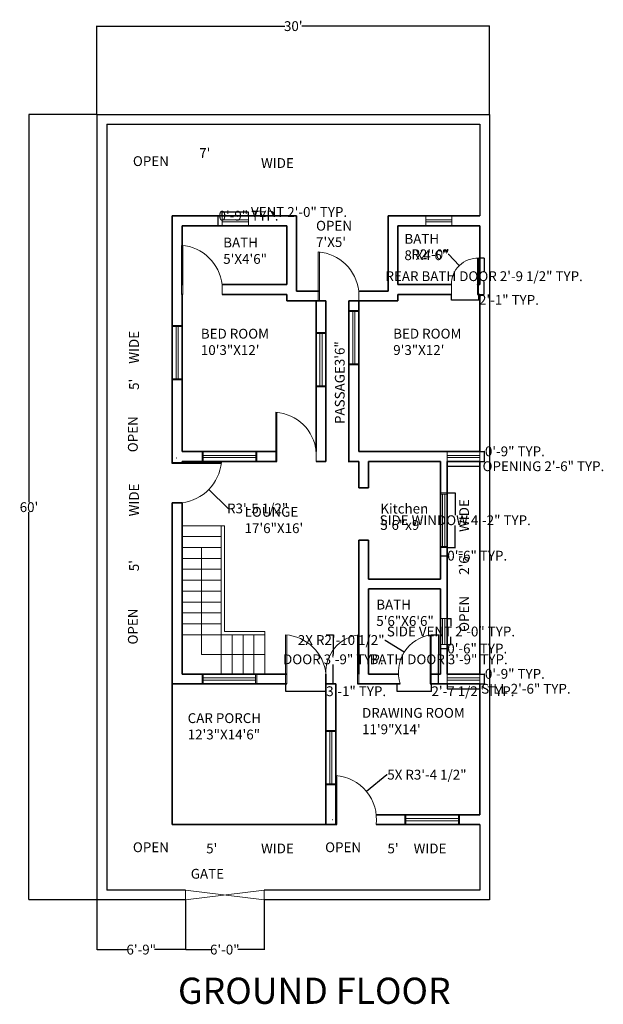
# Model space of a CAD drawing. Units: inches. Extents: x -56 to 1055, y -798 to 815.
# Tile 1 of 2: x -56 to 479, y -798 to 105. Entities that reach past the tile are written whole.
import ezdxf

# ---------------------------------------------------------------- set-up
doc = ezdxf.new("R2010")
doc.units = ezdxf.units.IN
doc.header["$MEASUREMENT"] = 0
for name, color, linetype, lineweight in [('A-ANNO-DIMS', 2, 'Continuous', 18), ('A-ANNO-TEXT', 7, 'Continuous', 18), ('A-AREA-IDEN', 7, 'Continuous', 18), ('A-DOOR', 3, 'Continuous', 18), ('A-FLOR-STRS', 7, 'Continuous', 18), ('A-GLAZ', 4, 'Continuous', 18), ('A-WALL', 7, 'Continuous', 35), ('C-PROP', 8, 'Continuous', 25), ('C-SITE-GATE', 3, 'Continuous', 18)]:
    doc.layers.add(name, color=color, linetype=linetype, lineweight=lineweight)
doc.styles.get("Standard").update_dxf_attribs({"font": 'arial.ttf'})
doc.dimstyles.get("Standard").update_dxf_attribs({"dimtxt": 9, "dimasz": 0.18, "dimexe": 0.18, "dimexo": 0.0625, "dimgap": 0.09, "dimtad": 0, "dimtih": 1, "dimtoh": 1, "dimdec": 0, "dimzin": 0, "dimdsep": 46, "dimlunit": 3, "dimtxsty": 'Standard', "dimcen": 0.09, "dimadec": 0, "dimazin": 0, "dimtfac": 1, "dimtdec": 0, "dimtofl": 0, "dimtmove": 0, "dimatfit": 3, "dimfxl": 1, "dimtolj": 1, "dimtzin": 0, "dimarcsym": 0})

# ---------------------------------------------------------------- blocks, each defined once
blk = doc.blocks.new('door')
for p, q in [((432.11, -633.03), (432.11, -588.03)), ((433.11, -633.03), (433.11, -588.03)), ((469.11, -624.03), (469.11, -633.03))]:
    blk.add_line(p, q)
blk.add_arc((428.9, -628.35), 40.45, 6.12759, 85.44206)
blk = doc.blocks.new('*D2')
at = {"layer": 'A-ANNO-DIMS', "color": 0, "lineweight": -2, "transparency": 16777216}
for p, q in [((15.17, 18.03), (15.17, 99.11)), ((15.35, 98.93), (187.44, 98.93)), ((374.99, 98.93), (202.89, 98.93)), ((375.17, 18.03), (375.17, 99.11))]:
    blk.add_line(p, q, dxfattribs=at)
at = {"layer": 'A-ANNO-DIMS', "color": 0, "transparency": 16777216}
for points in [[(15.35, 98.96), (15.35, 98.9), (15.17, 98.93)], [(374.99, 98.96), (374.99, 98.9), (375.17, 98.93)]]:
    blk.add_solid(points, dxfattribs=at)
at = {"layer": 'Defpoints', "color": 0, "transparency": 16777216}
for p in [(375.17, 98.93), (15.17, 17.97), (375.17, 17.97)]:
    blk.add_point(p, dxfattribs=at)
at = {"layer": 'A-ANNO-DIMS', "color": 0, "transparency": 16777216, "insert": (195.17, 98.93), "char_height": 9, "attachment_point": 5}
blk.add_mtext("\\A1;30'", dxfattribs=at)
blk = doc.blocks.new('*D3')
at = {"layer": 'A-ANNO-DIMS', "color": 0, "lineweight": -2, "transparency": 16777216}
for p, q in [((15.1, 17.97), (-47.33, 17.97)), ((-47.15, 17.79), (-47.15, -337.35)), ((-47.15, -701.85), (-47.15, -346.72)), ((15.1, -702.03), (-47.33, -702.03))]:
    blk.add_line(p, q, dxfattribs=at)
at = {"layer": 'A-ANNO-DIMS', "color": 0, "transparency": 16777216}
for points in [[(-47.18, 17.79), (-47.12, 17.79), (-47.15, 17.97)], [(-47.18, -701.85), (-47.12, -701.85), (-47.15, -702.03)]]:
    blk.add_solid(points, dxfattribs=at)
at = {"layer": 'Defpoints', "color": 0, "transparency": 16777216}
for p in [(-47.15, 17.97), (15.17, 17.97), (15.17, -702.03)]:
    blk.add_point(p, dxfattribs=at)
at = {"layer": 'A-ANNO-DIMS', "color": 0, "transparency": 16777216, "insert": (-47.15, -342.03), "char_height": 9, "attachment_point": 5}
blk.add_mtext("\\A1;60'", dxfattribs=at)
blk = doc.blocks.new('WIN-50-FRAMED')
for p, q in [((0, 50), (9, 50)), ((0, 0), (0, 50)), ((0, 49), (9, 49)), ((3.5, 1), (3.5, 49)), ((5.5, 1), (5.5, 49)), ((9, 0), (9, 50)), ((0, 1), (9, 1)), ((0, 0), (9, 0))]:
    blk.add_line(p, q)
blk = doc.blocks.new('WIN-50-JAMB')
for p, q in [((0, 0), (0, 9)), ((1, 0), (1, 9)), ((1, 5.5), (49, 5.5)), ((1, 3.5), (49, 3.5)), ((49, 0), (49, 9)), ((50, 0), (50, 9))]:
    blk.add_line(p, q)
blk = doc.blocks.new('WIN-50-NARROW-WALL')
for p, q in [((0, 50), (6, 50)), ((0, 49), (6, 49)), ((2, 49), (2, 1)), ((4, 49), (4, 1)), ((0, 1), (6, 1)), ((0, 0), (6, 0))]:
    blk.add_line(p, q)
blk = doc.blocks.new('WIN-24-NARROW-WALL')
for p, q in [((0, 24), (6, 24)), ((2, 24), (2, 0)), ((4, 24), (4, 0)), ((0, 0), (6, 0))]:
    blk.add_line(p, q)
blk = doc.blocks.new('WIN-24-VENT')
for p, q in [((0, 0), (0, 9)), ((0, 5.5), (24, 5.5)), ((0, 3.5), (24, 3.5)), ((24, 0), (24, 9))]:
    blk.add_line(p, q)
blk = doc.blocks.new('DOOR-BATH-FRONT')
for p, q in [((29.04, 0), (29.04, 45)), ((30.04, 0), (30.04, 45)), ((0.04, 9), (0.04, 12.42))]:
    blk.add_line(p, q)
blk.add_arc((34.59, 10.71), 34.59, 97.55718, 198.03398)
blk = doc.blocks.new('DOOR-BATH-REAR')
for p, q in [((24, 0), (24, 33.14)), ((25, 0), (25, 33.14)), ((0, 0), (0, 9.51))]:
    blk.add_line(p, q)
blk.add_arc((23.91, 9.26), 23.91, 87.38829, 180.61249)
blk = doc.blocks.new('DOOR-DRAWING-ROOM')
for p, q in [((29.04, 0), (29.04, 45)), ((30.04, 0), (30.04, 45))]:
    blk.add_line(p, q)
blk.add_arc((34.59, 10.71), 34.59, 97.55718, 182.83167)
blk = doc.blocks.new('STAIR-RETURN')
for p, q in [((36, 136), (0, 136)), ((36, 136), (36, 36)), ((36, 136), (39, 136)), ((39, 136), (39, 39)), ((36, 126), (0, 126)), ((36, 116), (0, 116)), ((18, 116), (18, 18)), ((36, 106), (0, 106)), ((36, 96), (0, 96)), ((36, 86), (0, 86)), ((36, 76), (0, 76)), ((36, 66), (0, 66)), ((36, 56), (0, 56)), ((36, 46), (0, 46)), ((76, 39), (39, 39)), ((76, 36), (76, 39)), ((36, 36), (0, 36)), ((76, 36), (36, 36)), ((36, 36), (36, 0)), ((46, 36), (46, 0)), ((56, 36), (56, 0)), ((66, 36), (66, 0)), ((76, 36), (76, 0)), ((18, 18), (76, 18))]:
    blk.add_line(p, q)
blk = doc.blocks.new('WIN-30-OPENING')
for p, q in [((0, 0), (0, 9)), ((0, 5.5), (30, 5.5)), ((0, 3.5), (30, 3.5)), ((30, 9), (30, 0))]:
    blk.add_line(p, q)
blk = doc.blocks.new('WIN-30-SILL')
for p, q in [((0, 0), (0, 9)), ((0, 5.5), (30, 5.5)), ((0, 3.5), (30, 3.5)), ((0, 0), (30, 0)), ((30, 9), (30, 0))]:
    blk.add_line(p, q)
blk = doc.blocks.new('*D17')
at = {"layer": 'A-ANNO-DIMS', "color": 0, "lineweight": -2, "transparency": 16777216}
for p, q in [((225.23, -459.03), (232.1, -459.03)), ((231.92, -459.21), (231.92, -476.78)), ((231.92, -503.85), (231.92, -486.28)), ((225.23, -504.03), (232.1, -504.03))]:
    blk.add_line(p, q, dxfattribs=at)
at = {"layer": 'A-ANNO-DIMS', "color": 0, "transparency": 16777216}
for points in [[(231.89, -459.21), (231.95, -459.21), (231.92, -459.03)], [(231.89, -503.85), (231.95, -503.85), (231.92, -504.03)]]:
    blk.add_solid(points, dxfattribs=at)
at = {"layer": 'Defpoints', "color": 0, "transparency": 16777216}
for p in [(225.17, -459.03), (231.92, -459.03), (225.17, -504.03)]:
    blk.add_point(p, dxfattribs=at)
at = {"layer": 'A-ANNO-DIMS', "color": 0, "transparency": 16777216, "insert": (231.92, -481.53), "char_height": 9, "attachment_point": 5}
blk.add_mtext('\\A1;DOOR 3\'-9" TYP.', dxfattribs=at)
blk = doc.blocks.new('*D18')
at = {"layer": 'A-ANNO-DIMS', "color": 0, "lineweight": -2, "transparency": 16777216}
for p, q in [((188.17, -504.09), (188.17, -510.96)), ((225.17, -504.09), (225.17, -510.96)), ((188.35, -510.78), (224.99, -510.78)), ((225.17, -510.78), (225.35, -510.78))]:
    blk.add_line(p, q, dxfattribs=at)
at = {"layer": 'A-ANNO-DIMS', "color": 0, "transparency": 16777216}
for points in [[(188.35, -510.75), (188.35, -510.81), (188.17, -510.78)], [(224.99, -510.75), (224.99, -510.81), (225.17, -510.78)]]:
    blk.add_solid(points, dxfattribs=at)
at = {"layer": 'Defpoints', "color": 0, "transparency": 16777216}
for p in [(188.17, -504.03), (225.17, -504.03), (225.17, -510.78)]:
    blk.add_point(p, dxfattribs=at)
at = {"layer": 'A-ANNO-DIMS', "color": 0, "transparency": 16777216, "insert": (252.86, -510.78), "char_height": 9, "attachment_point": 5}
blk.add_mtext('\\A1;3\'-1" TYP.', dxfattribs=at)
blk = doc.blocks.new('*D21')
at = {"layer": 'A-ANNO-DIMS', "color": 0, "lineweight": -2, "transparency": 16777216}
for p, q in [((130.04, -74.97), (130.04, -71.25)), ((130.22, -71.43), (153.86, -71.43)), ((154.04, -74.97), (154.04, -71.25)), ((154.04, -71.43), (154.22, -71.43))]:
    blk.add_line(p, q, dxfattribs=at)
at = {"layer": 'A-ANNO-DIMS', "color": 0, "transparency": 16777216}
for points in [[(130.22, -71.4), (130.22, -71.46), (130.04, -71.43)], [(153.86, -71.4), (153.86, -71.46), (154.04, -71.43)]]:
    blk.add_solid(points, dxfattribs=at)
at = {"layer": 'Defpoints', "color": 0, "transparency": 16777216}
for p in [(154.04, -71.43), (130.04, -75.03), (154.04, -75.03)]:
    blk.add_point(p, dxfattribs=at)
at = {"layer": 'A-ANNO-DIMS', "color": 0, "transparency": 16777216, "insert": (200.49, -71.43), "char_height": 9, "attachment_point": 5}
blk.add_mtext('\\A1;VENT 2\'-0" TYP.', dxfattribs=at)
blk = doc.blocks.new('*D22')
at = {"layer": 'A-ANNO-DIMS', "color": 0, "lineweight": -2, "transparency": 16777216}
for p, q in [((129.98, -75.03), (126.26, -75.03)), ((126.44, -75.03), (126.44, -74.85)), ((126.44, -74.85), (126.62, -74.85)), ((126.44, -83.85), (126.44, -75.21)), ((129.98, -84.03), (126.26, -84.03))]:
    blk.add_line(p, q, dxfattribs=at)
at = {"layer": 'A-ANNO-DIMS', "color": 0, "transparency": 16777216}
for points in [[(126.41, -75.21), (126.47, -75.21), (126.44, -75.03)], [(126.41, -83.85), (126.47, -83.85), (126.44, -84.03)]]:
    blk.add_solid(points, dxfattribs=at)
at = {"layer": 'Defpoints', "color": 0, "transparency": 16777216}
for p in [(126.44, -75.03), (130.04, -75.03), (130.04, -84.03)]:
    blk.add_point(p, dxfattribs=at)
at = {"layer": 'A-ANNO-DIMS', "color": 0, "transparency": 16777216, "insert": (154.14, -74.85), "char_height": 9, "attachment_point": 5}
blk.add_mtext('\\A1;0\'-9" TYP.', dxfattribs=at)
blk = doc.blocks.new('*D23')
at = {"layer": 'A-ANNO-DIMS', "color": 0, "lineweight": -2, "transparency": 16777216}
for p, q in [((336.23, -329.03), (343.85, -329.03)), ((343.67, -329.21), (343.67, -349.28)), ((343.67, -378.85), (343.67, -358.78)), ((336.23, -379.03), (343.85, -379.03))]:
    blk.add_line(p, q, dxfattribs=at)
at = {"layer": 'A-ANNO-DIMS', "color": 0, "transparency": 16777216}
for points in [[(343.64, -329.21), (343.7, -329.21), (343.67, -329.03)], [(343.64, -378.85), (343.7, -378.85), (343.67, -379.03)]]:
    blk.add_solid(points, dxfattribs=at)
at = {"layer": 'Defpoints', "color": 0, "transparency": 16777216}
for p in [(336.17, -329.03), (343.67, -329.03), (336.17, -379.03)]:
    blk.add_point(p, dxfattribs=at)
at = {"layer": 'A-ANNO-DIMS', "color": 0, "transparency": 16777216, "insert": (343.67, -354.03), "char_height": 9, "attachment_point": 5}
blk.add_mtext('\\A1;SIDE WINDOW 4\'-2" TYP.', dxfattribs=at)
blk = doc.blocks.new('*D24')
at = {"layer": 'A-ANNO-DIMS', "color": 0, "lineweight": -2, "transparency": 16777216}
for p, q in [((330.17, -379.09), (330.17, -386.71)), ((336.17, -379.09), (336.17, -386.71)), ((330.35, -386.53), (335.99, -386.53)), ((336.17, -386.53), (336.35, -386.53))]:
    blk.add_line(p, q, dxfattribs=at)
at = {"layer": 'A-ANNO-DIMS', "color": 0, "transparency": 16777216}
for points in [[(330.35, -386.5), (330.35, -386.56), (330.17, -386.53)], [(335.99, -386.5), (335.99, -386.56), (336.17, -386.53)]]:
    blk.add_solid(points, dxfattribs=at)
at = {"layer": 'Defpoints', "color": 0, "transparency": 16777216}
for p in [(330.17, -379.03), (336.17, -379.03), (336.17, -386.53)]:
    blk.add_point(p, dxfattribs=at)
at = {"layer": 'A-ANNO-DIMS', "color": 0, "transparency": 16777216, "insert": (363.87, -386.53), "char_height": 9, "attachment_point": 5}
blk.add_mtext('\\A1;0\'-6" TYP.', dxfattribs=at)
blk = doc.blocks.new('*D25')
at = {"layer": 'A-ANNO-DIMS', "color": 0, "lineweight": -2, "transparency": 16777216}
for p, q in [((336.23, -444.03), (339.95, -444.03)), ((339.77, -444.21), (339.77, -451.29)), ((336.23, -468.03), (339.95, -468.03)), ((339.77, -467.85), (339.77, -460.77))]:
    blk.add_line(p, q, dxfattribs=at)
at = {"layer": 'A-ANNO-DIMS', "color": 0, "transparency": 16777216}
for points in [[(339.74, -444.21), (339.8, -444.21), (339.77, -444.03)], [(339.74, -467.85), (339.8, -467.85), (339.77, -468.03)]]:
    blk.add_solid(points, dxfattribs=at)
at = {"layer": 'Defpoints', "color": 0, "transparency": 16777216}
for p in [(336.17, -444.03), (339.77, -444.03), (336.17, -468.03)]:
    blk.add_point(p, dxfattribs=at)
at = {"layer": 'A-ANNO-DIMS', "color": 0, "transparency": 16777216, "insert": (339.77, -456.03), "char_height": 9, "attachment_point": 5}
blk.add_mtext('\\A1;SIDE VENT 2\'-0" TYP.', dxfattribs=at)
blk = doc.blocks.new('*D26')
at = {"layer": 'A-ANNO-DIMS', "color": 0, "lineweight": -2, "transparency": 16777216}
for p, q in [((330.17, -468.09), (330.17, -471.81)), ((336.17, -468.09), (336.17, -471.81)), ((330.35, -471.63), (335.99, -471.63)), ((336.17, -471.63), (336.35, -471.63))]:
    blk.add_line(p, q, dxfattribs=at)
at = {"layer": 'A-ANNO-DIMS', "color": 0, "transparency": 16777216}
for points in [[(330.35, -471.6), (330.35, -471.66), (330.17, -471.63)], [(335.99, -471.6), (335.99, -471.66), (336.17, -471.63)]]:
    blk.add_solid(points, dxfattribs=at)
at = {"layer": 'Defpoints', "color": 0, "transparency": 16777216}
for p in [(330.17, -468.03), (336.17, -468.03), (336.17, -471.63)]:
    blk.add_point(p, dxfattribs=at)
at = {"layer": 'A-ANNO-DIMS', "color": 0, "transparency": 16777216, "insert": (363.87, -471.63), "char_height": 9, "attachment_point": 5}
blk.add_mtext('\\A1;0\'-6" TYP.', dxfattribs=at)
blk = doc.blocks.new('*D27')
at = {"layer": 'A-ANNO-DIMS', "color": 0, "lineweight": -2, "transparency": 16777216}
for p, q in [((321.74, -459.03), (328.61, -459.03)), ((328.43, -459.21), (328.43, -476.78)), ((328.43, -503.85), (328.43, -486.28)), ((321.74, -504.03), (328.61, -504.03))]:
    blk.add_line(p, q, dxfattribs=at)
at = {"layer": 'A-ANNO-DIMS', "color": 0, "transparency": 16777216}
for points in [[(328.4, -459.21), (328.46, -459.21), (328.43, -459.03)], [(328.4, -503.85), (328.46, -503.85), (328.43, -504.03)]]:
    blk.add_solid(points, dxfattribs=at)
at = {"layer": 'Defpoints', "color": 0, "transparency": 16777216}
for p in [(321.68, -459.03), (328.43, -459.03), (321.68, -504.03)]:
    blk.add_point(p, dxfattribs=at)
at = {"layer": 'A-ANNO-DIMS', "color": 0, "transparency": 16777216, "insert": (328.43, -481.53), "char_height": 9, "attachment_point": 5}
blk.add_mtext('\\A1;BATH DOOR 3\'-9" TYP.', dxfattribs=at)
blk = doc.blocks.new('*D28')
at = {"layer": 'A-ANNO-DIMS', "color": 0, "lineweight": -2, "transparency": 16777216}
for p, q in [((290.15, -504.09), (290.15, -510.96)), ((321.68, -504.09), (321.68, -510.96)), ((290.33, -510.78), (321.5, -510.78)), ((321.68, -510.78), (321.86, -510.78))]:
    blk.add_line(p, q, dxfattribs=at)
at = {"layer": 'A-ANNO-DIMS', "color": 0, "transparency": 16777216}
for points in [[(290.33, -510.75), (290.33, -510.81), (290.15, -510.78)], [(321.5, -510.75), (321.5, -510.81), (321.68, -510.78)]]:
    blk.add_solid(points, dxfattribs=at)
at = {"layer": 'Defpoints', "color": 0, "transparency": 16777216}
for p in [(290.15, -504.03), (321.68, -504.03), (321.68, -510.78)]:
    blk.add_point(p, dxfattribs=at)
at = {"layer": 'A-ANNO-DIMS', "color": 0, "transparency": 16777216, "insert": (359.94, -510.78), "char_height": 9, "attachment_point": 5}
blk.add_mtext('\\A1;2\'-7 1/2" TYP.', dxfattribs=at)
blk = doc.blocks.new('*D29')
at = {"layer": 'A-ANNO-DIMS', "color": 0, "lineweight": -2, "transparency": 16777216}
for p, q in [((365.24, -113.59), (370.37, -113.59)), ((370.19, -113.77), (370.19, -125.56)), ((370.19, -146.85), (370.19, -135.06)), ((365.24, -147.03), (370.37, -147.03))]:
    blk.add_line(p, q, dxfattribs=at)
at = {"layer": 'A-ANNO-DIMS', "color": 0, "transparency": 16777216}
for points in [[(370.16, -113.77), (370.22, -113.77), (370.19, -113.59)], [(370.16, -146.85), (370.22, -146.85), (370.19, -147.03)]]:
    blk.add_solid(points, dxfattribs=at)
at = {"layer": 'Defpoints', "color": 0, "transparency": 16777216}
for p in [(365.18, -113.59), (370.19, -113.59), (365.18, -147.03)]:
    blk.add_point(p, dxfattribs=at)
at = {"layer": 'A-ANNO-DIMS', "color": 0, "transparency": 16777216, "insert": (370.19, -130.31), "char_height": 9, "attachment_point": 5}
blk.add_mtext('\\A1;REAR BATH DOOR 2\'-9 1/2" TYP.', dxfattribs=at)
blk = doc.blocks.new('*D30')
at = {"layer": 'A-ANNO-DIMS', "color": 0, "lineweight": -2, "transparency": 16777216}
for p, q in [((340.11, -147.09), (340.11, -152.23)), ((340.29, -152.05), (365, -152.05)), ((365.18, -147.09), (365.18, -152.23)), ((365.18, -152.05), (365.36, -152.05))]:
    blk.add_line(p, q, dxfattribs=at)
at = {"layer": 'A-ANNO-DIMS', "color": 0, "transparency": 16777216}
for points in [[(340.29, -152.02), (340.29, -152.08), (340.11, -152.05)], [(365, -152.02), (365, -152.08), (365.18, -152.05)]]:
    blk.add_solid(points, dxfattribs=at)
at = {"layer": 'Defpoints', "color": 0, "transparency": 16777216}
for p in [(340.11, -147.03), (365.18, -147.03), (365.18, -152.05)]:
    blk.add_point(p, dxfattribs=at)
at = {"layer": 'A-ANNO-DIMS', "color": 0, "transparency": 16777216, "insert": (392.95, -152.05), "char_height": 9, "attachment_point": 5}
blk.add_mtext('\\A1;2\'-1" TYP.', dxfattribs=at)
blk = doc.blocks.new('*D35')
at = {"layer": 'A-ANNO-DIMS', "color": 0, "lineweight": -2, "transparency": 16777216}
for p, q in [((336.17, -300.09), (336.17, -304.71)), ((336.35, -304.53), (365.99, -304.53)), ((366.17, -300.09), (366.17, -304.71)), ((366.17, -304.53), (366.35, -304.53))]:
    blk.add_line(p, q, dxfattribs=at)
at = {"layer": 'A-ANNO-DIMS', "color": 0, "transparency": 16777216}
for points in [[(336.35, -304.5), (336.35, -304.56), (336.17, -304.53)], [(365.99, -304.5), (365.99, -304.56), (366.17, -304.53)]]:
    blk.add_solid(points, dxfattribs=at)
at = {"layer": 'Defpoints', "color": 0, "transparency": 16777216}
for p in [(336.17, -300.03), (366.17, -300.03), (366.17, -304.53)]:
    blk.add_point(p, dxfattribs=at)
at = {"layer": 'A-ANNO-DIMS', "color": 0, "transparency": 16777216, "insert": (424.56, -304.53), "char_height": 9, "attachment_point": 5}
blk.add_mtext('\\A1;OPENING 2\'-6" TYP.', dxfattribs=at)
blk = doc.blocks.new('*D36')
at = {"layer": 'A-ANNO-DIMS', "color": 0, "lineweight": -2, "transparency": 16777216}
for p, q in [((366.23, -291.03), (370.85, -291.03)), ((370.67, -291.03), (370.67, -290.85)), ((370.67, -290.85), (370.85, -290.85)), ((370.67, -299.85), (370.67, -291.21)), ((366.23, -300.03), (370.85, -300.03))]:
    blk.add_line(p, q, dxfattribs=at)
at = {"layer": 'A-ANNO-DIMS', "color": 0, "transparency": 16777216}
for points in [[(370.64, -291.21), (370.7, -291.21), (370.67, -291.03)], [(370.64, -299.85), (370.7, -299.85), (370.67, -300.03)]]:
    blk.add_solid(points, dxfattribs=at)
at = {"layer": 'Defpoints', "color": 0, "transparency": 16777216}
for p in [(366.17, -291.03), (370.67, -291.03), (366.17, -300.03)]:
    blk.add_point(p, dxfattribs=at)
at = {"layer": 'A-ANNO-DIMS', "color": 0, "transparency": 16777216, "insert": (398.37, -290.85), "char_height": 9, "attachment_point": 5}
blk.add_mtext('\\A1;0\'-9" TYP.', dxfattribs=at)
blk = doc.blocks.new('*D37')
at = {"layer": 'A-ANNO-DIMS', "color": 0, "lineweight": -2, "transparency": 16777216}
for p, q in [((336.17, -504.09), (336.17, -508.71)), ((366.17, -504.09), (366.17, -508.71)), ((336.35, -508.53), (365.99, -508.53)), ((366.17, -508.53), (366.35, -508.53))]:
    blk.add_line(p, q, dxfattribs=at)
at = {"layer": 'A-ANNO-DIMS', "color": 0, "transparency": 16777216}
for points in [[(336.35, -508.5), (336.35, -508.56), (336.17, -508.53)], [(365.99, -508.5), (365.99, -508.56), (366.17, -508.53)]]:
    blk.add_solid(points, dxfattribs=at)
at = {"layer": 'Defpoints', "color": 0, "transparency": 16777216}
for p in [(336.17, -504.03), (366.17, -504.03), (366.17, -508.53)]:
    blk.add_point(p, dxfattribs=at)
at = {"layer": 'A-ANNO-DIMS', "color": 0, "transparency": 16777216, "insert": (408.52, -508.53), "char_height": 9, "attachment_point": 5}
blk.add_mtext('\\A1;SILL 2\'-6" TYP.', dxfattribs=at)
blk = doc.blocks.new('*D38')
at = {"layer": 'A-ANNO-DIMS', "color": 0, "lineweight": -2, "transparency": 16777216}
for p, q in [((366.23, -495.03), (370.85, -495.03)), ((370.67, -495.03), (370.67, -494.85)), ((370.67, -494.85), (370.85, -494.85)), ((370.67, -503.85), (370.67, -495.21)), ((366.23, -504.03), (370.85, -504.03))]:
    blk.add_line(p, q, dxfattribs=at)
at = {"layer": 'A-ANNO-DIMS', "color": 0, "transparency": 16777216}
for points in [[(370.64, -495.21), (370.7, -495.21), (370.67, -495.03)], [(370.64, -503.85), (370.7, -503.85), (370.67, -504.03)]]:
    blk.add_solid(points, dxfattribs=at)
at = {"layer": 'Defpoints', "color": 0, "transparency": 16777216}
for p in [(366.17, -495.03), (370.67, -495.03), (366.17, -504.03)]:
    blk.add_point(p, dxfattribs=at)
at = {"layer": 'A-ANNO-DIMS', "color": 0, "transparency": 16777216, "insert": (398.37, -494.85), "char_height": 9, "attachment_point": 5}
blk.add_mtext('\\A1;0\'-9" TYP.', dxfattribs=at)
blk = doc.blocks.new('*D39')
at = {"layer": 'A-ANNO-DIMS', "color": 0, "lineweight": -2, "transparency": 16777216}
for p, q in [((15.17, -702.09), (15.17, -747.81)), ((96.4, -702.09), (96.4, -747.81)), ((15.35, -747.63), (43.7, -747.63)), ((96.22, -747.63), (67.86, -747.63))]:
    blk.add_line(p, q, dxfattribs=at)
at = {"layer": 'A-ANNO-DIMS', "color": 0, "transparency": 16777216}
for points in [[(15.35, -747.6), (15.35, -747.66), (15.17, -747.63)], [(96.22, -747.6), (96.22, -747.66), (96.4, -747.63)]]:
    blk.add_solid(points, dxfattribs=at)
at = {"layer": 'Defpoints', "color": 0, "transparency": 16777216}
for p in [(15.17, -702.03), (96.4, -702.03), (96.4, -747.63)]:
    blk.add_point(p, dxfattribs=at)
at = {"layer": 'A-ANNO-DIMS', "color": 0, "transparency": 16777216, "insert": (55.78, -747.63), "char_height": 9, "attachment_point": 5}
blk.add_mtext('\\A1;6\'-9"', dxfattribs=at)
blk = doc.blocks.new('*D40')
at = {"layer": 'A-ANNO-DIMS', "color": 0, "lineweight": -2, "transparency": 16777216}
for p, q in [((96.4, -702.09), (96.4, -747.81)), ((168.4, -702.09), (168.4, -747.81)), ((96.58, -747.63), (120.32, -747.63)), ((168.22, -747.63), (144.47, -747.63))]:
    blk.add_line(p, q, dxfattribs=at)
at = {"layer": 'A-ANNO-DIMS', "color": 0, "transparency": 16777216}
for points in [[(96.58, -747.6), (96.58, -747.66), (96.4, -747.63)], [(168.22, -747.6), (168.22, -747.66), (168.4, -747.63)]]:
    blk.add_solid(points, dxfattribs=at)
at = {"layer": 'Defpoints', "color": 0, "transparency": 16777216}
for p in [(96.4, -702.03), (168.4, -702.03), (168.4, -747.63)]:
    blk.add_point(p, dxfattribs=at)
at = {"layer": 'A-ANNO-DIMS', "color": 0, "transparency": 16777216, "insert": (132.4, -747.63), "char_height": 9, "attachment_point": 5}
blk.add_mtext('\\A1;6\'-0"', dxfattribs=at)
blk = doc.blocks.new('*D43')
at = {"layer": 'A-ANNO-DIMS', "color": 0, "lineweight": -2, "transparency": 16777216}
for p, q in [((87.87, -296.87), (88.05, -296.87)), ((87.96, -296.96), (87.96, -296.78)), ((135.49, -343.21), (117.8, -325.96)), ((135.67, -343.21), (135.49, -343.21))]:
    blk.add_line(p, q, dxfattribs=at)
at = {"layer": 'A-ANNO-DIMS', "color": 0, "transparency": 16777216}
blk.add_solid([(117.82, -325.93), (117.78, -325.98), (117.67, -325.83)], dxfattribs=at)
at = {"layer": 'Defpoints', "color": 0, "transparency": 16777216}
for p in [(87.96, -296.87), (117.67, -325.83)]:
    blk.add_point(p, dxfattribs=at)
at = {"layer": 'A-ANNO-DIMS', "color": 0, "transparency": 16777216, "insert": (162.52, -343.21), "char_height": 9, "attachment_point": 5}
blk.add_mtext('\\A1;R3\'-5 1/2"', dxfattribs=at)
blk = doc.blocks.new('*D44')
at = {"layer": 'A-ANNO-DIMS', "color": 0, "lineweight": -2, "transparency": 16777216}
for p, q in [((281.04, -587.28), (262.42, -602.56)), ((281.22, -587.28), (281.04, -587.28)), ((230.94, -628.35), (231.12, -628.35)), ((231.03, -628.44), (231.03, -628.26))]:
    blk.add_line(p, q, dxfattribs=at)
at = {"layer": 'A-ANNO-DIMS', "color": 0, "transparency": 16777216}
blk.add_solid([(262.4, -602.54), (262.44, -602.59), (262.28, -602.68)], dxfattribs=at)
at = {"layer": 'Defpoints', "color": 0, "transparency": 16777216}
for p in [(262.28, -602.68), (231.03, -628.35)]:
    blk.add_point(p, dxfattribs=at)
at = {"layer": 'A-ANNO-DIMS', "color": 0, "transparency": 16777216, "insert": (317.73, -587.28), "char_height": 9, "attachment_point": 5}
blk.add_mtext('\\A1;5X R3\'-4 1/2"', dxfattribs=at)
blk = doc.blocks.new('*D45')
at = {"layer": 'A-ANNO-DIMS', "color": 0, "lineweight": -2, "transparency": 16777216}
for p, q in [((279.22, -463.83), (279.4, -463.83)), ((279.4, -463.83), (296.81, -474.79)), ((326.14, -493.32), (326.32, -493.32)), ((326.23, -493.41), (326.23, -493.23))]:
    blk.add_line(p, q, dxfattribs=at)
at = {"layer": 'A-ANNO-DIMS', "color": 0, "transparency": 16777216}
blk.add_solid([(296.82, -474.77), (296.79, -474.82), (296.96, -474.89)], dxfattribs=at)
at = {"layer": 'Defpoints', "color": 0, "transparency": 16777216}
for p in [(296.96, -474.89), (326.23, -493.32)]:
    blk.add_point(p, dxfattribs=at)
at = {"layer": 'A-ANNO-DIMS', "color": 0, "transparency": 16777216, "insert": (239.13, -463.83), "char_height": 9, "attachment_point": 5}
blk.add_mtext('\\A1;2X R2\'-10 1/2"', dxfattribs=at)
blk = doc.blocks.new('*D46')
at = {"layer": 'A-ANNO-DIMS', "color": 0, "lineweight": -2, "transparency": 16777216}
for p, q in [((337.33, -110.25), (337.51, -110.25)), ((337.51, -110.25), (347.35, -120.45)), ((364, -137.78), (364.18, -137.78)), ((364.09, -137.87), (364.09, -137.69))]:
    blk.add_line(p, q, dxfattribs=at)
at = {"layer": 'A-ANNO-DIMS', "color": 0, "transparency": 16777216}
blk.add_solid([(347.37, -120.42), (347.33, -120.47), (347.48, -120.57)], dxfattribs=at)
at = {"layer": 'Defpoints', "color": 0, "transparency": 16777216}
for p in [(347.48, -120.57), (364.09, -137.78)]:
    blk.add_point(p, dxfattribs=at)
at = {"layer": 'A-ANNO-DIMS', "color": 0, "transparency": 16777216, "insert": (320.97, -110.25), "char_height": 9, "attachment_point": 5}
blk.add_mtext('\\A1;R2\'-0"', dxfattribs=at)

msp = doc.modelspace()

# ---------------------------------------------------------------- linework, layer by layer
at = {"layer": 'A-DOOR'}
for p, q in [((84.17, -301.03), (129.24, -301.03)), ((84.17, -302.03), (129.24, -302.03)), ((234.24, -633.03), (234.24, -588.03)), ((235.24, -633.03), (235.24, -588.03))]:
    msp.add_line(p, q, dxfattribs=at)
for centre, radius, start, end in [((87.96, -296.87), 41.49, 277.20755, 354.24269), ((231.03, -628.35), 40.45, 353.35134, 85.44206)]:
    msp.add_arc(centre, radius, start, end, dxfattribs=at)
at = {"layer": 'A-WALL'}
for p, q in [((84.17, -75.03), (198.17, -75.03)), ((84.17, -75.03), (84.17, -302.03)), ((198.17, -75.03), (198.17, -144.03)), ((282.17, -75.03), (282.17, -144.03)), ((282.17, -75.03), (366.17, -75.03)), ((93.17, -84.03), (189.17, -84.03)), ((93.17, -84.03), (93.17, -138.03)), ((189.17, -84.03), (189.17, -138.03)), ((291.17, -84.03), (291.17, -138.03)), ((291.17, -84.03), (366.17, -84.03)), ((366.17, -84.03), (366.17, -138.03)), ((93.17, -138.03), (93.85, -138.03)), ((129.85, -138.03), (189.17, -138.03)), ((198.17, -144.03), (219.17, -144.03)), ((255.17, -144.03), (282.17, -144.03)), ((291.17, -138.03), (340.18, -138.03)), ((366.17, -138.03), (365.18, -137.89)), ((365.18, -138.03), (366.17, -138.03)), ((93.17, -147.03), (93.85, -147.03)), ((93.17, -147.03), (93.17, -291.03)), ((129.85, -147.03), (189.17, -147.03)), ((189.17, -147.03), (189.17, -153.03)), ((189.17, -153.03), (225.17, -153.03)), ((216.17, -153.03), (216.17, -291.03)), ((225.17, -153.03), (225.17, -300.03)), ((246.17, -153.03), (291.17, -153.03)), ((246.17, -153.03), (246.17, -300.03)), ((255.17, -153.03), (255.17, -291.03)), ((255.17, -153.03), (267.17, -153.03)), ((291.17, -147.03), (340.18, -147.03)), ((291.17, -153.03), (291.17, -147.03)), ((364.18, -147.03), (366.17, -147.03)), ((366.17, -147.03), (366.17, -291.03)), ((93.17, -291.03), (180.26, -291.03)), ((255.17, -291.03), (366.17, -291.03)), ((93.17, -300.03), (180.26, -300.03)), ((93.17, -300.03), (93.17, -302.03)), ((93.17, -300.03), (93.24, -301.03)), ((216.26, -300.03), (225.17, -300.03)), ((255.17, -300.03), (245.5, -300.03)), ((255.17, -300.03), (255.17, -324.29)), ((267.17, -300.03), (264.17, -300.03)), ((264.17, -300.03), (264.17, -324.29)), ((267.17, -300.03), (330.17, -300.03)), ((330.17, -300.03), (330.17, -408.03)), ((336.17, -300.03), (336.17, -417.03)), ((336.17, -300.03), (366.17, -300.03)), ((366.17, -300.03), (366.17, -495.03)), ((264.17, -324.29), (255.17, -324.29)), ((84.17, -338.03), (93.17, -338.03)), ((84.17, -338.03), (84.17, -633.03)), ((93.17, -338.03), (93.17, -495.03)), ((264.17, -372.29), (255.17, -372.29)), ((255.17, -372.29), (255.17, -495.03)), ((264.17, -372.29), (264.17, -408.03)), ((264.17, -408.03), (330.17, -408.03)), ((264.17, -417.03), (330.17, -417.03)), ((264.17, -417.03), (264.17, -495.03)), ((330.17, -417.03), (330.17, -495.03)), ((336.17, -417.03), (336.17, -495.03)), ((189.17, -495.03), (93.17, -495.03)), ((225.17, -495.03), (225.17, -633.03)), ((264.17, -495.03), (291.68, -495.03)), ((321.68, -495.03), (330.17, -495.03)), ((336.17, -495.03), (366.17, -495.03)), ((189.17, -504.03), (84.17, -504.03)), ((234.17, -504.03), (225.17, -504.03)), ((234.17, -504.03), (234.17, -633.03)), ((255.17, -504.03), (254.17, -504.03)), ((255.17, -504.03), (293.34, -504.03)), ((320.68, -504.03), (366.17, -504.03)), ((366.17, -504.03), (366.17, -624.03)), ((225.17, -624.03), (225.17, -588.03)), ((366.17, -624.03), (271.24, -624.03)), ((235.24, -633.03), (84.17, -633.03)), ((366.17, -633.03), (271.2, -633.03))]:
    msp.add_line(p, q, dxfattribs=at)
at = {"layer": 'C-PROP'}
for p, q in [((15.17, 17.97), (375.17, 17.97)), ((15.17, 17.97), (15.17, -702.03)), ((375.17, 17.97), (375.17, -702.03)), ((24.17, 8.97), (24.17, -693.03)), ((24.17, 8.97), (366.17, 8.97)), ((366.17, 8.97), (366.17, -75.03)), ((366.17, -633.03), (366.17, -693.03)), ((96.4, -693.03), (24.17, -693.03)), ((366.17, -693.03), (168.4, -693.03)), ((96.4, -702.03), (15.17, -702.03)), ((375.17, -702.03), (168.4, -702.03))]:
    msp.add_line(p, q, dxfattribs=at)
at = {"layer": 'C-SITE-GATE'}
for p, q in [((96.4, -693.03), (96.4, -702.03)), ((96.4, -702.03), (168.4, -693.03)), ((168.4, -702.03), (96.4, -693.03)), ((168.4, -693.03), (168.4, -702.03))]:
    msp.add_line(p, q, dxfattribs=at)

# ---------------------------------------------------------------- block references
at = {"layer": 'A-DOOR'}
for name, p in [('door', (-339.26, 486)), ('door', (-213.95, 480)), ('DOOR-BATH-REAR', (340.18, -147.03)), ('door', (-252.86, 333)), ('door', (-243.95, 129)), ('DOOR-DRAWING-ROOM', (225.12, -504.03)), ('DOOR-BATH-FRONT', (291.64, -504.03))]:
    msp.add_blockref(name, p, dxfattribs=at)
at = {"layer": 'A-FLOR-STRS'}
msp.add_blockref('STAIR-RETURN', (93.17, -495.03), dxfattribs=at)
at = {"layer": 'A-GLAZ'}
for name, p in [('WIN-24-VENT', (130.04, -84.03)), ('WIN-24-VENT', (316.67, -84.03)), ('WIN-50-FRAMED', (246.17, -211.71)), ('WIN-50-FRAMED', (84.17, -225.44)), ('WIN-50-FRAMED', (216.17, -231.86)), ('WIN-50-JAMB', (111.71, -300.03)), ('WIN-30-OPENING', (336.17, -300.03)), ('WIN-50-NARROW-WALL', (330.17, -379.03)), ('WIN-24-NARROW-WALL', (330.17, -468.03)), ('WIN-50-JAMB', (111.67, -504.03)), ('WIN-30-SILL', (336.17, -504.03))]:
    msp.add_blockref(name, p, dxfattribs=at)
for name, p, rotation in [('WIN-50-JAMB', (225.17, -546.67), 269.9999999999998), ('WIN-50-FRAMED', (297.54, -624.03), 269.9999999999993)]:
    msp.add_blockref(name, p, dxfattribs=dict(at, rotation=rotation))

# ---------------------------------------------------------------- texts
at = {"layer": 'A-ANNO-TEXT', "attachment_point": 1}
for s, width, insert, char_height in [("7'", 30.8214, (108.92, -12.91), 9), ('OPEN', 37.4235, (48.14, -20.32), 9), ('WIDE', 49.2396, (165.64, -22.07), 9), ('OPEN', 37.4235, (48.14, -649.32), 9), ('OPEN', 37.4235, (224.4, -649.32), 9), ("5'", 46.6759, (115.32, -650.41), 9), ('WIDE', 49.2396, (165.64, -650.4), 9), ("5'", 46.6759, (281.56, -650.41), 9), ('WIDE', 49.2396, (305.55, -650.4), 9), ('GATE', 64.625, (101.2, -673.63), 9), ('\\pxt0;GROUND FLOOR', 379.4894, (89.48, -773.37), 24)]:
    msp.add_mtext_dynamic_manual_height_columns(s, width=width, gutter_width=1, heights=[0], dxfattribs=dict(at, insert=insert, char_height=char_height))
at = {"layer": 'A-ANNO-TEXT', "char_height": 9, "attachment_point": 1, "rotation": 90}
for s, width, insert in [('WIDE', 49.2396, (44.67, -210.54)), ("5'", 46.6759, (44.68, -234.53)), ('OPEN', 37.4235, (43.59, -291.69)), ('WIDE', 49.2396, (44.67, -350.45)), ('OPEN       2\'6"      WIDE', 153.2574, (347.33, -456.39)), ("5'", 46.6759, (44.68, -400.77)), ('OPEN', 37.4235, (43.59, -467.95))]:
    msp.add_mtext_dynamic_manual_height_columns(s, width=width, gutter_width=1, heights=[0], dxfattribs=dict(at, insert=insert))
at = {"layer": 'A-AREA-IDEN', "char_height": 9, "attachment_point": 1}
for s, width, insert in [("OPEN\\P7'X5'", 55.271, (216.08, -79.54)), ('BATH\\P5\'X4\'6"', 73.9291, (130.97, -94.98)), ('BATH\\P8\'X4\'6"', 57.336, (297.11, -91.59)), ('BED ROOM\\P10\'3"X12\'', 86.6235, (110.46, -178.53)), ('BED ROOM\\P9\'3"X12\'', 63.0941, (286.84, -178.48)), ('LOUNGE\\P17\'6"X16\'', 92.9805, (150.55, -341.82)), ('Kitchen\\P5\'6"x9\'', 50.4169, (275, -338.86)), ('BATH\\P5\'6"X6\'6"', 45.2259, (271.29, -426.88)), ('CAR PORCH\\P12\'3"X14\'6"', 108.4659, (98.36, -530.96)), ('DRAWING ROOM\\P11\'9"X14\'', 98.021, (258.25, -526.15))]:
    msp.add_mtext_dynamic_manual_height_columns(s, width=width, gutter_width=1, heights=[0], dxfattribs=dict(at, insert=insert))
at = {"layer": 'A-AREA-IDEN', "insert": (233.32, -265.82), "char_height": 9, "attachment_point": 1, "rotation": 90}
msp.add_mtext_dynamic_manual_height_columns('PASSAGE3\'6"', width=12.3522, gutter_width=1, heights=[0], dxfattribs=at)

# ---------------------------------------------------------------- dimensions: what is measured, and where the dimension line sits
at = {"layer": 'A-ANNO-DIMS'}
for base, p1, p2, override, picture, middle in [((375.17, 98.93), (15.17, 17.97), (375.17, 17.97), {"dimclrd": 0, "dimclre": 0, "dimclrt": 0}, '*D2', (195.17, 98.93)), ((96.4, -747.63), (15.17, -702.03), (96.4, -702.03), {"dimdec": 1, "dimlfac": 1, "dimrnd": 0, "dimzin": 1, "dimdsep": 46, "dimlunit": 4, "dimfrac": 2}, '*D39', (55.78, -747.63)), ((168.4, -747.63), (96.4, -702.03), (168.4, -702.03), {"dimdec": 1, "dimlfac": 1, "dimrnd": 0, "dimzin": 1, "dimdsep": 46, "dimlunit": 4, "dimfrac": 2}, '*D40', (132.4, -747.63))]:
    dim = msp.add_linear_dim(base=base, p1=p1, p2=p2, dimstyle='Standard', override=override, dxfattribs=at)
    dim.commit()
    dim.dimension.update_dxf_attribs({"geometry": picture, "text_midpoint": middle})
dim = msp.add_linear_dim(base=(-47.15, 17.97), p1=(15.17, -702.03), p2=(15.17, 17.97), angle=270, dimstyle='Standard', override={"dimclrd": 0, "dimclre": 0, "dimclrt": 0}, dxfattribs=at)
dim.commit()
dim.dimension.update_dxf_attribs({"geometry": '*D3', "text_midpoint": (-47.15, -342.03)})
for base, p1, p2, text, picture, middle in [((154.04, -71.43), (130.04, -75.03), (154.04, -75.03), 'VENT <> TYP.', '*D21', (200.49, -71.43)), ((365.18, -152.05), (340.11, -147.03), (365.18, -147.03), '<> TYP.', '*D30', (392.95, -152.05)), ((366.17, -304.53), (336.17, -300.03), (366.17, -300.03), 'OPENING <> TYP.', '*D35', (424.56, -304.53)), ((336.17, -386.53), (330.17, -379.03), (336.17, -379.03), '<> TYP.', '*D24', (363.87, -386.53)), ((336.17, -471.63), (330.17, -468.03), (336.17, -468.03), '<> TYP.', '*D26', (363.87, -471.63)), ((321.68, -510.78), (290.15, -504.03), (321.68, -504.03), '<> TYP.', '*D28', (359.94, -510.78)), ((366.17, -508.53), (336.17, -504.03), (366.17, -504.03), 'SILL <> TYP.', '*D37', (408.52, -508.53)), ((225.17, -510.78), (188.17, -504.03), (225.17, -504.03), '<> TYP.', '*D18', (252.86, -510.78))]:
    dim = msp.add_linear_dim(base=base, p1=p1, p2=p2, text=text, dimstyle='Standard', override={"dimdec": 1, "dimlfac": 1, "dimrnd": 0, "dimzin": 1, "dimdsep": 46, "dimlunit": 4, "dimfrac": 2}, dxfattribs=at)
    dim.commit()
    dim.dimension.update_dxf_attribs({"geometry": picture, "text_midpoint": middle})
for base, p1, p2, text, picture, middle in [((126.44, -75.03), (130.04, -84.03), (130.04, -75.03), '<> TYP.', '*D22', (154.14, -74.85)), ((370.19, -113.59), (365.18, -147.03), (365.18, -113.59), 'REAR BATH DOOR <> TYP.', '*D29', (370.19, -130.31)), ((370.67, -291.03), (366.17, -300.03), (366.17, -291.03), '<> TYP.', '*D36', (398.37, -290.85)), ((343.67, -329.03), (336.17, -379.03), (336.17, -329.03), 'SIDE WINDOW <> TYP.', '*D23', (343.67, -354.03)), ((339.77, -444.03), (336.17, -468.03), (336.17, -444.03), 'SIDE VENT <> TYP.', '*D25', (339.77, -456.03)), ((231.92, -459.03), (225.17, -504.03), (225.17, -459.03), 'DOOR <> TYP.', '*D17', (231.92, -481.53)), ((328.43, -459.03), (321.68, -504.03), (321.68, -459.03), 'BATH DOOR <> TYP.', '*D27', (328.43, -481.53)), ((370.67, -495.03), (366.17, -504.03), (366.17, -495.03), '<> TYP.', '*D38', (398.37, -494.85))]:
    dim = msp.add_linear_dim(base=base, p1=p1, p2=p2, angle=90, text=text, dimstyle='Standard', override={"dimdec": 1, "dimlfac": 1, "dimrnd": 0, "dimzin": 1, "dimdsep": 46, "dimlunit": 4, "dimfrac": 2}, dxfattribs=at)
    dim.commit()
    dim.dimension.update_dxf_attribs({"geometry": picture, "text_midpoint": middle})
for center, mpoint, picture, middle in [((364.09, -137.78), (347.48, -120.57), '*D46', (320.97, -110.25)), ((87.96, -296.87), (117.67, -325.83), '*D43', (162.52, -343.21))]:
    dim = msp.add_radius_dim(center=center, mpoint=mpoint, dimstyle='Standard', override={"dimdec": 1, "dimlfac": 1, "dimrnd": 0, "dimzin": 1, "dimdsep": 46, "dimlunit": 4, "dimfrac": 2}, dxfattribs=at)
    dim.commit()
    dim.dimension.update_dxf_attribs({"geometry": picture, "text_midpoint": middle, "dimtype": 164})
for center, mpoint, text, picture, middle in [((326.23, -493.32), (296.96, -474.89), '2X <>', '*D45', (239.13, -463.83)), ((231.03, -628.35), (262.28, -602.68), '5X <>', '*D44', (317.73, -587.28))]:
    dim = msp.add_radius_dim(center=center, mpoint=mpoint, text=text, dimstyle='Standard', override={"dimdec": 1, "dimlfac": 1, "dimrnd": 0, "dimzin": 1, "dimdsep": 46, "dimlunit": 4, "dimfrac": 2}, dxfattribs=at)
    dim.commit()
    dim.dimension.update_dxf_attribs({"geometry": picture, "text_midpoint": middle, "dimtype": 164})

doc.saveas('drawing.dxf')
